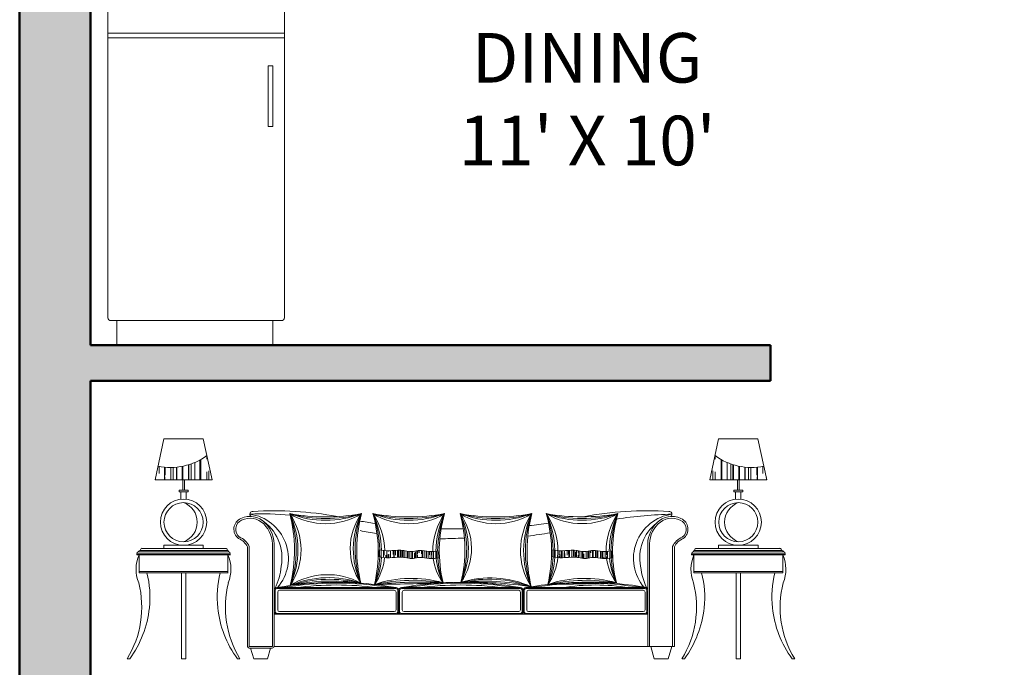
# Model space of a CAD drawing. Units: inches. Extents: x 1771 to 3025, y 319 to 889.
# Tile 7 of 35: x 1800 to 1939, y 713 to 805. Entities that reach past the tile are written whole.
import ezdxf

# ---------------------------------------------------------------- set-up
doc = ezdxf.new("R2010")
doc.units = ezdxf.units.IN
doc.header["$MEASUREMENT"] = 0
doc.set_wipeout_variables(frame=1)
for name, color, linetype, lineweight in [('A-AREA-IDEN', 241, 'Continuous', 25), ('A-FURN', 8, 'Continuous', 18), ('A-WALL', 7, 'Continuous', 50), ('A-WALL-PATT', 254, 'Continuous', 13)]:
    doc.layers.add(name, color=color, linetype=linetype, lineweight=lineweight)
doc.styles.get("Standard").update_dxf_attribs({"font": 'arial.ttf'})

# ---------------------------------------------------------------- blocks, each defined once
blk = doc.blocks.new('A$C301F3DA3')
for p, q in [((156.7, 1006), (206.7, 1236)), ((206.7, 1236), (427.8, 1236)), ((477.8, 1006), (427.8, 1236)), ((3275.4, 1006), (3325.4, 1236)), ((3546.5, 1236), (3325.4, 1236)), ((3596.5, 1006), (3546.5, 1236)), ((409.5, 1006), (409.5, 1117.6)), ((411, 1006), (411, 1118.4)), ((414, 1006), (414, 1120.1)), ((447.5, 1121.4), (447.5, 1141.6)), ((3305.7, 1121.4), (3305.7, 1141.6)), ((3339.2, 1006), (3339.2, 1120.1)), ((3342.2, 1006), (3342.2, 1118.4)), ((3343.7, 1006), (3343.7, 1117.6)), ((179.5, 1041.4), (179.5, 1081.1)), ((209.5, 1006), (209.5, 1076.8)), ((211.5, 1060.9), (211.5, 1076.6)), ((213, 1031.4), (213, 1076.5)), ((246.5, 1006), (246.5, 1075.2)), ((259.5, 1006), (259.5, 1075.6)), ((278, 1006), (278, 1073.4)), ((280, 1006), (280, 1077.1)), ((309.5, 1006), (309.5, 1081.6)), ((313.5, 1006), (313.5, 1082.4)), ((344.5, 1006), (344.5, 1090.3)), ((347, 1006), (347, 1091.1)), ((359.5, 1006), (359.5, 1095.2)), ((380.5, 1006), (380.5, 1103.5)), ((459.5, 1006), (459.5, 1056.4)), ((3293.7, 1006), (3293.7, 1056.4)), ((3372.7, 1006), (3372.7, 1103.5)), ((3393.7, 1006), (3393.7, 1095.2)), ((3406.2, 1006), (3406.2, 1091.1)), ((3408.7, 1006), (3408.7, 1090.3)), ((3439.7, 1006), (3439.7, 1082.4)), ((3443.7, 1006), (3443.7, 1081.6)), ((3473.2, 1006), (3473.2, 1077.1)), ((3475.2, 1006), (3475.2, 1073.4)), ((3493.7, 1006), (3493.7, 1075.6)), ((3506.7, 1006), (3506.7, 1075.2)), ((3540.2, 1031.4), (3540.2, 1076.5)), ((3541.7, 1060.9), (3541.7, 1076.6)), ((3543.7, 1006), (3543.7, 1076.8)), ((3573.7, 1041.4), (3573.7, 1081.1)), ((156.7, 1006), (477.8, 1006)), ((159.5, 1006), (159.5, 1019)), ((211.5, 1006), (211.5, 1023.4)), ((312.2, 948), (312.2, 1006)), ((322.2, 948), (322.2, 1006)), ((322.2, 948), (322.2, 1006)), ((447.5, 1006), (447.5, 1051.4)), ((477.5, 1006), (477.5, 1007.2)), ((3596.5, 1006), (3275.4, 1006)), ((3275.7, 1006), (3275.7, 1007.2)), ((3305.7, 1006), (3305.7, 1051.4)), ((3431, 948), (3431, 1006)), ((3431, 948), (3431, 1006)), ((3441, 948), (3441, 1006)), ((3541.7, 1006), (3541.7, 1023.4)), ((3593.7, 1006), (3593.7, 1019)), ((292.2, 938), (292.2, 948)), ((342.2, 948), (292.2, 948)), ((342.2, 938), (342.2, 948)), ((3411, 938), (3411, 948)), ((3411, 948), (3461, 948)), ((3461, 938), (3461, 948)), ((342.2, 938), (292.2, 938)), ((302.2, 896.9), (302.2, 938)), ((332.2, 896.9), (332.2, 938)), ((3411, 938), (3461, 938)), ((3421, 896.9), (3421, 938)), ((3451, 896.9), (3451, 938)), ((557.5, 620.8), (82.9, 620.8)), ((206.3, 637.8), (428.1, 637.8)), ((206.3, 637.8), (206.3, 620.8)), ((428.1, 637.8), (428.1, 620.8)), ((3195.6, 620.8), (3670.3, 620.8)), ((3546.9, 637.8), (3325, 637.8)), ((3325, 637.8), (3325, 620.8)), ((3546.9, 637.8), (3546.9, 620.8)), ((53.7, 590.8), (53.7, 584.4)), ((67.1, 584.4), (67.1, 484)), ((565.7, 608.8), (75.3, 608.8)), ((557.5, 608.8), (82.9, 608.8)), ((566.3, 584.4), (566.3, 484)), ((3186.9, 584.4), (3186.9, 484)), ((3187.5, 608.8), (3677.9, 608.8)), ((3195.6, 608.8), (3670.3, 608.8)), ((3686.1, 584.4), (3686.1, 484)), ((3699.5, 590.8), (3699.5, 584.4)), ((567.3, 490), (67.1, 490)), ((567.3, 484), (67.1, 484)), ((305.2, 484), (305.2, 0)), ((329.2, 484), (329.2, 0)), ((3185.9, 490), (3686.1, 490)), ((3185.9, 484), (3686.1, 484)), ((3424, 484), (3424, 0)), ((3448, 484), (3448, 0)), ((0, 0), (14.7, 0)), ((329.2, 0), (305.2, 0)), ((3424, 0), (3448, 0)), ((3753.2, 0), (3738.4, 0))]:
    blk.add_line(p, q)
for centre, radius in [((317.2, 767.8), 130), ((3436, 767.8), 130), ((317.2, 767.8), 110), ((3436, 767.8), 110)]:
    blk.add_circle(centre, radius)
for centre, radius, start, end in [((243.2, 1422.6), 347.4, 258.3829, 306.1467), ((3510, 1422.6), 347.4, 233.8533, 281.6171), ((276.7, 767.8), 117.2, 290.217, 69.783), ((3476.5, 767.8), 117.2, 110.217, 249.783), ((86.1, 609.2), 12.1, 105.2269, 181.3736), ((551.7, 609.3), 12.5, 357.6342, 66.9804), ((3201.5, 609.3), 12.5, 113.0196, 182.3658), ((3667.1, 609.2), 12.1, 358.6264, 74.7731), ((250.8, 503.3), 200.8, 156.1653, 202.3822), ((63.8, 591), 10.1, 100.6467, 181.1131), ((74, 595.7), 13.1, 84.2874, 156.7847), ((561.8, 599.3), 9.8, 9.6184, 76.537), ((3191.3, 599.3), 9.8, 103.463, 170.3816), ((3679.2, 595.7), 13.1, 23.2153, 95.7126), ((3502.4, 503.3), 200.8, 337.6178, 23.8347), ((3689.4, 591), 10.1, 358.8869, 79.3533), ((-428.9, 346.4), 557.3, 353.825, 14.2983), ((1063.3, 346.4), 557.3, 165.7017, 186.175), ((2689.9, 346.4), 557.3, 353.825, 14.2983), ((4182.1, 346.4), 557.3, 165.7017, 186.175), ((-472, 290.4), 554.2, 328.3965, 14.2533), ((4225.2, 290.4), 554.2, 165.7467, 211.6035), ((-467.1, 350.3), 595.7, 323.9815, 353.8447), ((4220.2, 350.3), 595.7, 186.1553, 216.0185)]:
    blk.add_arc(centre, radius, start, end)
blk.add_wipeout([(3041.8, 0), (2963.5, 0), (2943.5, 70), (826.6, 70), (824.2, 65.5), (819.2, 61.4), (815.3, 60), (806.8, 60), (789.7, 0), (711.4, 0), (694.3, 60), (685.4, 60), (681.9, 61.7), (678.1, 65.9), (676.6, 70), (676.6, 628.7), (667.5, 644), (650.9, 661.4), (635.1, 671.5), (625.4, 676.3), (610.1, 693.4), (602.5, 710.5), (600.1, 728.4), (604.2, 751.4), (623, 778.5), (639.5, 788.9), (669, 798), (689.6, 799.7), (696.6, 800), (691.2, 806.8), (690.2, 814.9), (693.8, 823.2), (701.1, 828), (705.9, 828.8), (865.5, 832), (984.1, 825.9), (1111.6, 811), (1170.7, 801.2), (1180.3, 799.4), (1231.4, 803.5), (1293.2, 811.6), (1317.6, 815.8), (1310.3, 786.3), (1307.6, 774.2), (1389.8, 761.2), (1393.6, 767.5), (1388.1, 790.9), (1381.5, 815.8), (1418.2, 809.7), (1480.9, 802.2), (1546.1, 798.2), (1588.9, 797.6), (1683.4, 802), (1730, 807.2), (1784.7, 815.8), (1774.6, 776.7), (1767.8, 744), (1769.2, 730.8), (1890.2, 730.7), (1884.7, 761.4), (1877, 795.8), (1871.7, 815.8), (1919.1, 808.2), (1966.4, 802.7), (2026, 798.6), (2073.3, 797.6), (2145.9, 799.9), (2221.5, 807.4), (2273.8, 815.4), (2267.3, 783.6), (2260.5, 748.2), (2369.1, 762), (2361.7, 794), (2355.9, 815.8), (2402.1, 808.4), (2442.8, 803.5), (2477.3, 800.5), (2535.4, 797.9), (2572.4, 797.9), (2610.4, 806.1), (2648.6, 812), (2670.2, 815.1), (2740.7, 823.3), (2819.6, 829.3), (2905.4, 832.2), (2981.5, 831.5), (3045.3, 828.6), (3053.9, 827.3), (3059.6, 822.9), (3062.8, 816.3), (3062.9, 810.1), (3060.6, 804.3), (3056.6, 800), (3070.6, 799.5), (3085.9, 797.7), (3105.1, 792.4), (3120.7, 785.3), (3134.4, 774.5), (3143.7, 762.3), (3150.7, 746.2), (3153, 725.9), (3150.1, 708.7), (3142.9, 693.1), (3133.2, 681), (3126.6, 675.3), (3114.9, 669.8), (3100.2, 659.6), (3082.1, 638.7), (3076.6, 628.7), (3076.6, 70), (3061.8, 70)])
for p, q in [((3056.6, 800), (3056.6, 799.5)), ((676.6, 70), (676.6, 628.7)), ((686.6, 70), (686.6, 630.8)), ((816.6, 70), (816.6, 647.2)), ((826.6, 70), (826.6, 627.7)), ((2926.6, 70), (2926.6, 647.2)), ((2936.6, 70), (2936.6, 647.2)), ((3066.6, 70), (3066.6, 630.8)), ((3076.6, 70), (3076.6, 628.7)), ((580.7, 590.8), (53.7, 590.8)), ((580.7, 584.4), (53.7, 584.4)), ((61.9, 600.9), (572.5, 600.9)), ((579.7, 590.8), (579.7, 584.4)), ((3172.5, 590.8), (3699.5, 590.8)), ((3172.5, 584.4), (3699.5, 584.4)), ((3173.5, 590.8), (3173.5, 584.4)), ((3691.3, 600.9), (3180.7, 600.9)), ((826.6, 400), (826.6, 265)), ((1511.6, 400), (841.6, 400)), ((1511.2, 395), (841.6, 395)), ((1541.6, 400), (2211.6, 400)), ((1542, 395), (2211.2, 395)), ((2241.6, 400), (2911.6, 400)), ((2242, 395), (2911.2, 395)), ((846.6, 275), (846.6, 375)), ((856.6, 385), (1501.6, 385)), ((1511.6, 375), (1511.6, 275)), ((1526.6, 265), (1526.6, 385)), ((1526.6, 265), (1526.6, 385)), ((1531.6, 265.4), (1531.6, 384.6)), ((1546.6, 275), (1546.6, 375)), ((1556.6, 385), (2201.6, 385)), ((2211.6, 375), (2211.6, 275)), ((2221.6, 384.6), (2221.6, 265.4)), ((2226.6, 265), (2226.6, 385)), ((2226.6, 385), (2226.6, 265)), ((2231.6, 265.4), (2231.6, 384.6)), ((2246.6, 275), (2246.6, 375)), ((2256.6, 385), (2901.6, 385)), ((2911.6, 375), (2911.6, 275)), ((2921.6, 384.6), (2921.6, 265.4)), ((1511.6, 250), (826.6, 250)), ((2926.6, 250), (826.6, 250)), ((841.6, 250), (1511.6, 250)), ((842, 255), (1511.6, 255)), ((1501.6, 265), (856.6, 265)), ((2211.6, 255), (1542, 255)), ((2201.6, 265), (1556.6, 265)), ((2911.2, 255), (2242, 255)), ((2901.6, 265), (2256.6, 265)), ((685.4, 60), (815.3, 60)), ((686.6, 70), (816.6, 70)), ((711.4, 0), (694.3, 60)), ((806.8, 60), (789.7, 0)), ((2926.6, 70), (826.6, 70)), ((2926.6, 70), (3076.6, 70)), ((3061.8, 70), (2943.5, 70)), ((2943.5, 70), (2963.5, 0)), ((3041.8, 0), (3061.8, 70)), ((633.4, 0), (618.7, 0)), ((789.7, 0), (711.4, 0)), ((2963.5, 0), (3041.8, 0)), ((3119.8, 0), (3134.5, 0))]:
    blk.add_line(p, q)
at = {"ltscale": 0.1}
for p, q in [((1418.8, 573), (1418.8, 612.1)), ((1427.8, 571.6), (1427.8, 610.7)), ((1440.6, 576.7), (1440.6, 609)), ((1508.2, 582.7), (1508.2, 609.5)), ((1520.6, 571.3), (1520.6, 610.4)), ((1521.6, 571.4), (1521.6, 610.5)), ((1525.2, 571.5), (1525.2, 610.6)), ((1535, 571.6), (1535, 610.7)), ((1540.6, 571.3), (1540.6, 610.4)), ((1548.4, 570.6), (1548.4, 609.6)), ((1551.8, 570.1), (1551.8, 609.2)), ((1642.2, 594.7), (1642.2, 609)), ((1655.6, 590.7), (1655.6, 609.3)), ((1658.2, 608.3), (1658.2, 609.1)), ((2392.6, 573.1), (2392.6, 610.7)), ((2400.6, 571.9), (2400.6, 610.9)), ((2403, 571.5), (2403, 610.6)), ((2406, 571.1), (2406, 610.1)), ((2480.6, 588.7), (2480.6, 609.3)), ((2482.8, 570.4), (2482.8, 609.5)), ((2486.4, 570.7), (2486.4, 609.8)), ((2499.8, 571.5), (2499.8, 610.6)), ((2500.6, 571.5), (2500.6, 610.7)), ((2509.4, 576.9), (2509.4, 610.7)), ((2513.2, 571.4), (2513.2, 610.5)), ((2526.6, 570.1), (2526.6, 609.1)), ((2620.4, 590.7), (2620.4, 609.3)), ((2620.6, 570.2), (2620.6, 609.3)), ((2633.8, 570), (2633.8, 609)), ((1414.4, 573.7), (1414.4, 606.7)), ((1420.6, 572.7), (1420.6, 580.7)), ((1441.2, 569.8), (1441.2, 608.9)), ((1445.4, 583.3), (1445.4, 608.4)), ((1454.6, 568.5), (1454.6, 582.7)), ((1460.6, 568.1), (1460.6, 607.2)), ((1468, 606.7), (1468, 607)), ((1468, 567.8), (1468, 586.7)), ((1472, 603.3), (1472, 606.9)), ((1472, 567.8), (1472, 588.3)), ((1480.6, 568.1), (1480.6, 588.7)), ((1481.4, 568.1), (1481.4, 607.3)), ((1494.8, 586.7), (1494.8, 608.3)), ((1498.6, 569.5), (1498.6, 608.3)), ((1500.6, 569.7), (1500.6, 608.8)), ((1560.6, 568.8), (1560.6, 607.9)), ((1561.8, 568.6), (1561.8, 607.7)), ((1575.2, 566.4), (1575.2, 605.5)), ((1578.4, 565.9), (1578.4, 605)), ((1580.6, 565.6), (1580.6, 604.7)), ((1588.6, 564.6), (1588.6, 603.7)), ((1600.6, 564), (1600.6, 603.1)), ((1602, 564), (1602, 590.7)), ((1605, 568.3), (1605, 603.3)), ((1615.4, 565.2), (1615.4, 594.7)), ((1620.6, 566.1), (1620.6, 600.7)), ((1628.8, 567.7), (1628.8, 606.9)), ((1631.6, 588.3), (1631.6, 607.4)), ((1631.6, 568.2), (1631.6, 581.7)), ((1640.6, 596.7), (1640.6, 608.8)), ((1655.6, 570.2), (1655.6, 570.7)), ((1658.2, 570), (1658.2, 601.7)), ((1660.6, 569.8), (1660.6, 608.9)), ((1669, 568.8), (1669, 607.9)), ((1680.6, 566.9), (1680.6, 606)), ((1682.4, 570.7), (1682.4, 605.7)), ((1684.8, 566.2), (1684.8, 605.3)), ((1695.8, 566.7), (1695.8, 603.7)), ((1700.6, 584.7), (1700.6, 603.2)), ((1700.6, 564.1), (1700.6, 564.7)), ((1709.2, 563.6), (1709.2, 602.7)), ((1711.4, 581.7), (1711.4, 602.7)), ((1711.4, 563.6), (1711.4, 566.7)), ((1720.6, 563.7), (1720.6, 602.8)), ((1722.6, 563.7), (1722.6, 602.9)), ((1736, 564.6), (1736, 603.8)), ((1738, 601.7), (1738, 603.9)), ((1738, 564.8), (1738, 586.7)), ((1740.6, 565), (1740.6, 604.2)), ((1749.4, 565.9), (1749.4, 598.7)), ((2419.4, 569.4), (2419.4, 582.7)), ((2420.6, 569.2), (2420.6, 608.3)), ((2429.6, 583.5), (2429.6, 607.5)), ((2429.6, 568.4), (2429.6, 576.9)), ((2432.8, 606.7), (2432.8, 607.3)), ((2432.8, 568.2), (2432.8, 586.7)), ((2440.6, 567.9), (2440.6, 607)), ((2446.2, 567.8), (2446.2, 606.9)), ((2456.2, 603.5), (2456.2, 607.3)), ((2456.2, 568.1), (2456.2, 596.9)), ((2459.6, 586.7), (2459.6, 607.5)), ((2460.6, 568.4), (2460.6, 592.7)), ((2473, 582.7), (2473, 608.6)), ((2520.6, 570.8), (2520.6, 600.7)), ((2536, 596.9), (2536, 607.7)), ((2536, 568.6), (2536, 581.9)), ((2540, 568), (2540, 607)), ((2540.6, 576.7), (2540.6, 606.9)), ((2553.4, 565.8), (2553.4, 604.9)), ((2560.6, 564.9), (2560.6, 604)), ((2562.6, 564.7), (2562.6, 601.9)), ((2566.8, 564.3), (2566.8, 590.7)), ((2580.2, 564.2), (2580.2, 594.7)), ((2580.6, 564.2), (2580.6, 603.3)), ((2589.2, 565.2), (2589.2, 604.3)), ((2593.6, 565.9), (2593.6, 605.1)), ((2600.6, 567.2), (2600.6, 606.4)), ((2607, 594.7), (2607, 607.6)), ((2615.8, 569.8), (2615.8, 608.9)), ((2620.4, 570.2), (2620.4, 570.7)), ((2640.6, 569.2), (2640.6, 608.3)), ((2642.4, 569), (2642.4, 608)), ((2647.2, 570.7), (2647.2, 607.3)), ((2660.6, 566), (2660.6, 605.1)), ((2660.6, 566.7), (2660.6, 605.1)), ((2669, 564.8), (2669, 603.8)), ((2674, 564.2), (2674, 603.3)), ((2680.6, 563.8), (2680.6, 568.7)), ((2687.4, 563.6), (2687.4, 602.7)), ((2695.6, 581.9), (2695.6, 602.8)), ((2695.6, 563.7), (2695.6, 575.3)), ((2700.6, 564.7), (2700.6, 603.1)), ((2700.8, 563.9), (2700.8, 603.1)), ((2714.2, 565), (2714.2, 598.7)), ((2720.6, 565.6), (2720.6, 604.8)), ((2722.2, 601.9), (2722.2, 604.9)), ((2722.2, 565.8), (2722.2, 595.3)), ((2727.6, 566.4), (2727.6, 602.7))]:
    blk.add_line(p, q, dxfattribs=at)
at = {"ltscale": 0.2}
for p, q in [((831.6, 384.6), (831.6, 265.4)), ((1521.6, 265.4), (1521.6, 384.6))]:
    blk.add_line(p, q, dxfattribs=at)
for centre, radius, start, end in [((826.9, -1080.6), 1912.9, 79.3535, 93.5671), ((2926.5, -1083.7), 1916.1, 86.4466, 100.8971), ((666.4, 728.4), 66.3, 113.9424, 233.1116), ((666.4, 728.4), 56.3, 113.9424, 233.1116), ((689.6, 677.8), 121.9, 45.5351, 114.264), ((689.6, 677.8), 111.9, 45.5351, 114.264), ((705.9, 812.9), 15.9, 82.93, 233.9986), ((118.5, 608.8), 822.4, 346.1538, 14.5736), ((1116, 1923.3), 1125.7, 259.6832, 280.3168), ((2062.3, 614.6), 771.4, 164.8808, 194.229), ((611.7, 598.3), 800, 346.9565, 15.7738), ((1583.1, 1923.3), 1125.7, 259.6832, 280.3168), ((2517.6, 605.2), 762.6, 163.9697, 193.489), ((2073.3, 1923.3), 1125.7, 259.6832, 280.3168), ((1147.1, 613.7), 752.3, 345.8635, 15.5852), ((3098.6, 604.6), 850.3, 165.6218, 193.5679), ((2556.6, 1923.4), 1125.7, 259.7316, 280.3651), ((1586.1, 598.3), 800, 346.9565, 15.7738), ((3493.3, 605.3), 763.9, 163.9835, 193.4773), ((3063.6, 677.8), 121.9, 65.736, 134.4649), ((3063.6, 677.8), 111.9, 65.736, 134.4649), ((3047.3, 812.9), 15.9, 306.0014, 97.07), ((3086.8, 728.4), 56.3, 306.8884, 66.0576), ((3086.8, 728.4), 66.3, 306.8884, 66.0576), ((647.8, 638.7), 169.2, 356.5069, 44.7501), ((647.8, 638.7), 179.2, 356.5069, 44.7501), ((1820.4, 3753.3), 3022.9, 260.2329, 261.8106), ((1820.4, 3753.3), 3022.9, 269.0301, 271.0652), ((1932.8, 3753.3), 3022.9, 268.9348, 269.193), ((1932.8, 3753.3), 3022.9, 276.2234, 278.2985), ((3105.4, 638.7), 179.2, 135.2499, 176.5069), ((3105.4, 638.7), 169.2, 135.2499, 183.4931), ((593.4, 589.7), 91.9, 24.952, 68.8167), ((593.4, 589.7), 101.9, 23.8355, 68.8167), ((3159.8, 589.7), 101.9, 112.0106, 156.1645), ((3159.8, 589.7), 91.9, 111.1833, 155.048), ((382.6, 503.3), 200.8, 337.6178, 23.8347), ((562.8, 585.5), 17.7, 17.558, 60.6823), ((3370.5, 503.3), 200.8, 156.1653, 202.3822), ((3190.4, 585.5), 17.7, 119.3177, 162.442), ((1106.4, 290.4), 554.2, 165.7467, 211.6035), ((844.1, 382.5), 17.7, 98.1301, 171.8699), ((844.1, 382.5), 12.7, 101.3731, 171.8699), ((1176.6, -1455.4), 1885.4, 79.7654, 100.2346), ((1150.7, -658.8), 1096, 81.404, 102.3155), ((1256.5, 13610.3), 13193.2, 270.58435, 272.25734), ((1509.1, 382.5), 12.7, 9.6036, 81.8699), ((1509.1, 382.5), 17.7, 8.1301, 81.8699), ((1544.1, 382.5), 17.7, 98.1301, 171.8699), ((1544.1, 382.5), 12.7, 99.6036, 170.3964), ((1876.6, -1455.4), 1885.4, 79.7654, 100.2346), ((1933.3, -1830.3), 2260.9, 81.3836, 91.4369), ((2209.1, 382.5), 12.7, 9.6036, 81.8699), ((2209.1, 382.5), 17.7, 8.1301, 81.8699), ((2244.1, 382.5), 17.7, 98.1301, 171.8699), ((2244.1, 382.5), 12.7, 98.1301, 170.3964), ((2584.1, -1540.1), 1970.1, 79.9883, 100.0117), ((2230.8, 13610.3), 13193.2, 270.58435, 272.25734), ((2909.1, 382.5), 12.7, 9.6036, 80.3964), ((2909.1, 382.5), 17.7, 8.1301, 81.8699), ((2646.8, 290.4), 554.2, 328.3965, 14.2533), ((856.6, 375), 10, 90, 180), ((1501.6, 375), 10, 0, 90), ((1556.6, 375), 10, 90, 180), ((2201.6, 375), 10, 0, 90), ((2256.6, 375), 10, 90, 180), ((2901.6, 375), 10, 0, 90), ((1101.5, 350.3), 595.7, 186.1553, 216.0185), ((2651.7, 350.3), 595.7, 323.9815, 353.8447), ((844.1, 267.5), 17.7, 188.1301, 261.8699), ((844.1, 267.5), 12.7, 189.6036, 260.3964), ((856.6, 275), 10, 180, 270), ((1501.6, 275), 10, 270, 0), ((1509.1, 267.5), 12.7, 278.1301, 351.8699), ((1509.1, 267.5), 17.7, 278.1301, 351.8699), ((1544.1, 267.5), 17.7, 188.1301, 261.8699), ((1544.1, 267.5), 12.7, 188.1301, 261.8699), ((1556.6, 275), 10, 180, 270), ((2201.6, 275), 10, 270, 0), ((2209.1, 267.5), 12.7, 278.1301, 350.3964), ((2209.1, 267.5), 17.7, 278.1301, 351.8699), ((2244.1, 267.5), 17.7, 188.1301, 261.8699), ((2244.1, 267.5), 12.7, 189.6036, 261.8699), ((2256.6, 275), 10, 180, 270), ((2901.6, 275), 10, 270, 0), ((2909.1, 267.5), 12.7, 278.1301, 350.3964), ((2909.1, 267.5), 17.7, 278.1301, 351.8699), ((689.4, 72.4), 13, 190.4691, 252.2297), ((812.4, 74.7), 15, 281.33, 341.8376)]:
    blk.add_arc(centre, radius, start, end)
for centre, radius, start, end in [((760.4, -701.1), 1515.6, 84.0764, 92.659), ((655.5, 564.2), 251.1, 319.4042, 82.0915), ((615.4, 566.9), 255.3, 349.3926, 57.2195), ((478.9, 611.1), 481.1, 335.5564, 25.171), ((347.1, 610.3), 603.3, 340.8164, 19.911), ((617, 612), 360.5, 326.3119, 34.4155), ((1116, 1147.7), 388.4, 238.7274, 301.2726), ((1116, 1532.7), 744.8, 254.2902, 285.613), ((1116.1, 1337.7), 559.4, 249.0479, 290.9906), ((1594, 618.2), 339.8, 144.4467, 214.6631), ((1723.9, 617.2), 452.3, 153.955, 205.1549), ((1847.8, 616.2), 566.5, 159.3751, 199.7347), ((757.4, 589.8), 663.8, 1.8995, 19.9071), ((904.2, 593.4), 526.6, 1.8365, 24.977), ((1057.3, 597.5), 390.8, 1.5581, 33.948), ((1583.1, 1147.7), 388.4, 238.7274, 301.2726), ((1583.2, 1532.7), 744.8, 254.2902, 285.613), ((1583.2, 1337.7), 559.4, 249.0479, 290.9906), ((2089.5, 604.3), 371, 145.2427, 180.2355), ((2233.6, 600.8), 497.7, 154.4139, 179.665), ((2371.5, 597.7), 626, 159.6139, 179.3615), ((2073.3, 1147.7), 388.4, 238.7274, 301.2726), ((2073.4, 1532.7), 744.8, 254.2902, 285.613), ((1604, 619.4), 332, 325.1926, 36.2561), ((1356.4, 616.3), 552.6, 340.2903, 21.1584), ((1477.2, 617.8), 441.4, 334.806, 26.6427), ((2073.4, 1337.7), 559.4, 249.0479, 290.9906), ((2583.5, 608.3), 371.9, 146.084, 213.1057), ((2726, 607.2), 497, 155.1926, 203.9971), ((2862.3, 606.3), 623.6, 160.3704, 198.8193), ((2557.2, 1147.9), 388.4, 238.7757, 301.3209), ((1731.8, 589.8), 663.8, 1.8995, 19.9071), ((1878.6, 593.4), 526.6, 1.8365, 24.977), ((2031.7, 597.5), 390.8, 1.5581, 33.948), ((2556.9, 1532.9), 744.8, 254.3386, 285.6614), ((2557.2, 1337.9), 559.4, 249.0965, 291.0392), ((3065, 604.3), 372, 145.2936, 180.2364), ((3209.5, 600.8), 499.2, 154.453, 179.666), ((3347.8, 597.7), 627.9, 159.6457, 179.3628), ((3116.2, -1577.3), 2390.8, 91.2711, 98.7869), ((3097.7, 564.2), 251.1, 97.9085, 220.5958), ((1756.4, 2902), 2227.1, 258.4292, 260.8447), ((3129.1, 568.5), 247.1, 128.4831, 191.3403), ((1756.4, 2902), 2227.1, 270.0938, 273.071), ((1995, 2902), 2227.1, 266.929, 267.4707), ((1995, 2902), 2227.1, 276.6418, 279.9147), ((902.9, 592.1), 518.2, 340.3477, 357.8599), ((1016.3, 594.9), 414.5, 334.6941, 356.7301), ((1135.5, 598), 312.7, 324.8043, 354.7159), ((2016.9, 603.5), 298.4, 187.6695, 216.1919), ((2130.5, 600.8), 394.6, 185.2441, 206.0823), ((2238.4, 598.3), 492.9, 183.7951, 200.2933), ((1877.3, 592.1), 518.2, 340.3477, 357.8599), ((1990.7, 594.9), 414.5, 334.6941, 356.7301), ((2109.9, 598), 312.7, 324.8043, 354.7159), ((2991.3, 603.5), 298.4, 187.6695, 216.1919), ((3104.9, 600.8), 394.6, 185.2441, 206.0823), ((3212.8, 598.3), 492.9, 183.7951, 200.2933), ((468.9, 563.6), 399.8, 334.9958, 353.7174), ((3284.3, 563.6), 399.8, 186.2826, 206.5398), ((1126.7, 81.6), 391.4, 61.3182, 122.4012), ((1138.5, -278.6), 725.3, 76.0429, 107.785), ((1132.5, -88.7), 544.9, 70.6018, 113.1041), ((1599, -199.4), 651.3, 74.2187, 108.623), ((2041.7, -102.7), 557.6, 65.6014, 107.2191), ((2031.9, -256.9), 704.2, 70.1587, 102.7402), ((2573.4, -199.4), 651.3, 74.2187, 108.623), ((1176.6, -1429.1), 1854.1, 80.5803, 99.4197), ((1176.6, -1342.3), 1757.3, 82.5085, 97.4915), ((1646.2, -2030.8), 2461.8, 87.001, 95.9502), ((1608.6, -583.8), 1025.1, 80.6601, 102.1611), ((1876.6, -1429.1), 1854.1, 80.5803, 99.4197), ((1876.6, -1429.1), 1844.1, 82.6871, 97.3129), ((2004.4, -699.8), 1137, 76.444, 96.455), ((2584.1, -1521.2), 1946.2, 80.8066, 99.1934), ((2620.6, -2030.8), 2461.8, 87.001, 95.9502), ((2583, -583.8), 1025.1, 80.6601, 102.1611), ((2634.1, -753.4), 1168.4, 80.809, 99.191)]:
    blk.add_arc(centre, radius, start, end, dxfattribs=at)
for points in [[(1411.2, 613.3), (1432, 609.9), (1474.4, 603.1), (1540.1, 616.4), (1597.7, 597.2), (1650.5, 614.1), (1699.8, 599.6), (1736.2, 603.6), (1755.3, 605.7)], [(2385.5, 613.3), (2406.4, 609.9), (2448.8, 603.1), (2514.5, 616.4), (2572, 597.2), (2624.9, 614.1), (2674.2, 599.6), (2710.6, 603.6), (2729.6, 605.7)], [(1411.5, 574.2), (1432.4, 570.8), (1474.8, 564), (1540.5, 577.3), (1598, 558.1), (1650.9, 575), (1700.2, 560.5), (1736.6, 564.5), (1755.6, 566.6)], [(2385.9, 574.2), (2406.8, 570.8), (2449.2, 564), (2514.8, 577.3), (2572.4, 558.1), (2625.2, 575), (2674.5, 560.5), (2711, 564.5), (2730, 566.6)]]:
    blk.add_open_spline(points, degree=3, knots=[0, 0, 0, 0, 62.941123, 128.023226, 196.918691, 236.354413, 288.676993, 345.703861, 345.703861, 345.703861, 345.703861])
blk = doc.blocks.new('A$C43BC2F3A')
for p, q in [((0, 1490.5), (0, 93.5)), ((10, 1500), (590, 1500)), ((600, 1490), (600, 93.5)), ((590, 83.5), (10.3, 83.5)), ((22.6, 83.5), (561, 83.5)), ((30.8, 0), (30.8, 83.5)), ((561, 83.5), (561, 0)), ((561, 0), (30.8, 0))]:
    blk.add_line(p, q)
for points in [[(561, 1344.2), (561, 1188.3), (544.3, 1188.3), (544.3, 1344.2)], [(561, 949), (561, 743), (544.3, 743), (544.3, 949)]]:
    blk.add_lwpolyline(points, close=True)
for points in [[(600, 1060.3), (0, 1060.3)], [(600, 1043.6), (0, 1043.6)]]:
    blk.add_lwpolyline(points)
for centre, radius, start, end in [((10, 1490), 10, 90, 180), ((590, 1490), 10, 0, 90), ((10.5, 94), 10.5, 182.8791, 268.8051), ((590, 93.5), 10, 270, 0)]:
    blk.add_arc(centre, radius, start, end)

msp = doc.modelspace()

# ---------------------------------------------------------------- hatches: boundary and pattern name
at = {"layer": 'A-WALL-PATT'}
h = msp.add_hatch(color=256, dxfattribs=at)
h.dxf.hatch_style = 1
h.paths.add_polyline_path([(1870.72, 888.63), (1799.72, 888.63), (1799.72, 878.63), (1870.72, 878.63)])
h.paths.add_polyline_path([(1968.77, 888.63), (1918.72, 888.63), (1918.72, 878.63), (1941.72, 878.63), (1941.72, 830.63), (1946.72, 830.63), (1946.72, 878.63), (1968.77, 878.63)])
h.paths.add_polyline_path([(2059.68, 888.63), (2016.77, 888.63), (2016.77, 878.63), (2037.72, 878.63), (2037.72, 794.63), (1941.72, 794.63), (1941.72, 758.63), (1941.72, 664.63), (1946.72, 664.63), (1946.72, 712), (1946.72, 789.63), (2054.72, 789.63), (2054.72, 794.63), (2042.33, 794.63), (2042.33, 798.62), (2042.33, 835.5), (2042.72, 878.63), (2059.68, 878.63)])
h.paths.add_polyline_path([(2100.72, 888.63), (2077.68, 888.63), (2077.68, 878.63), (2090.72, 878.63), (2090.72, 789.63), (2090.72, 768.61), (2100.72, 768.61)])
h.paths.add_polyline_path([(2100.72, 720.61), (2090.72, 720.61), (2090.72, 669.63), (1982.72, 669.63), (1982.72, 664.63), (2001.72, 664.63), (2001.72, 652.63), (2006.72, 652.63), (2006.72, 664.63), (2049.52, 664.63, -0.385549), (2050.52, 664.63), (2090.72, 664.63), (2090.72, 649.17), (2100.72, 649.17)])
edge = h.paths.add_edge_path()
edge.add_line((2100.72, 631.17), (2090.72, 631.17))
edge.add_line((2090.72, 631.17), (2090.72, 616.63))
edge.add_line((2090.72, 616.63), (2001.72, 616.63))
edge.add_line((2001.72, 616.63), (1982.72, 616.63))
edge.add_line((1982.72, 616.63), (1982.72, 611.63))
edge.add_line((1982.72, 611.63), (2024.67, 611.63))
edge.add_spline(control_points=[(2024.67, 611.63), (2027.58, 612.87), (2030.01, 613.31), (2032.47, 613.72)], knot_values=[484.321569, 484.321569, 484.321569, 484.321569, 625.498764, 625.498764, 625.498764, 625.498764], degree=3, periodic=0)
edge.add_line((2032.47, 613.72), (2033.2, 613.72))
edge.add_spline(control_points=[(2033.2, 613.72), (2035.66, 613.31), (2039.46, 612.87), (2042.2, 611.63)], knot_values=[484.321569, 484.321569, 484.321569, 484.321569, 625.498764, 625.498764, 625.498764, 625.498764], degree=3, periodic=0)
edge.add_line((2042.2, 611.63), (2090.72, 611.63))
edge.add_line((2090.72, 611.63), (2090.72, 581.11))
edge.add_line((2090.72, 581.11), (2100.72, 581.11))
edge.add_line((2100.72, 581.11), (2100.72, 631.17))
h.paths.add_polyline_path([(2100.72, 533.11), (2090.72, 533.11), (2090.72, 479.63), (1946.72, 479.63), (1946.72, 616.63), (1936.72, 616.63), (1936.72, 543.63), (1845.72, 543.63), (1845.72, 533.63), (1936.72, 533.63), (1936.72, 469.63), (2090.72, 469.63), (2090.72, 452.76), (2100.72, 452.76)])
h.paths.add_polyline_path([(2100.72, 404.76), (2090.72, 404.76), (2090.72, 393.63), (1936.72, 393.63), (1936.72, 383.63), (2100.72, 383.63)])
h.paths.add_polyline_path([(1905.72, 758.63), (1835.47, 758.63), (1835.47, 758.63), (1813.44, 758.63), (1809.72, 758.63), (1809.72, 842.59, -0.008336), (1808.42, 842.63), (1799.72, 842.63), (1799.72, 690.58), (1809.72, 690.58), (1809.72, 753.63), (1905.72, 753.63)])
h.paths.add_polyline_path([(1809.72, 642.58), (1799.72, 642.58), (1799.72, 533.63), (1809.72, 533.63), (1809.72, 581)])

# ---------------------------------------------------------------- linework, layer by layer
at = {"layer": 'A-WALL'}
for p, q in [((1799.72, 842.63), (1799.72, 533.63)), ((1809.72, 842.63), (1809.72, 758.63)), ((1905.72, 758.63), (1809.72, 758.63)), ((1905.72, 758.63), (1905.72, 753.63)), ((1905.72, 753.63), (1809.72, 753.63)), ((1809.72, 753.63), (1809.72, 533.63))]:
    msp.add_line(p, q, dxfattribs=at)

# ---------------------------------------------------------------- block references
at = {"layer": 'A-FURN', "xscale": 0.0415387277892195, "yscale": 0.0415387277892195, "zscale": 0.0415387277892195}
msp.add_blockref('A$C43BC2F3A', (1812.17, 758.63), dxfattribs=at)

# ---------------------------------------------------------------- texts
at = {"layer": 'A-AREA-IDEN', "insert": (1837.09, 802.68), "char_height": 7, "attachment_point": 1}
msp.add_mtext_dynamic_manual_height_columns("\\pxqc;DINING \\P11' X 10'", width=85.4611, gutter_width=1, heights=[0], dxfattribs=at)

# ---------------------------------------------------------------- next in the draw order: block references
at = {"layer": 'A-FURN', "xscale": 0.0251055470835414, "yscale": 0.0251055470835414, "zscale": 0.0251055470835414}
msp.add_blockref('A$C301F3DA3', (1814.89, 714.39), dxfattribs=at)

doc.saveas('drawing.dxf')
